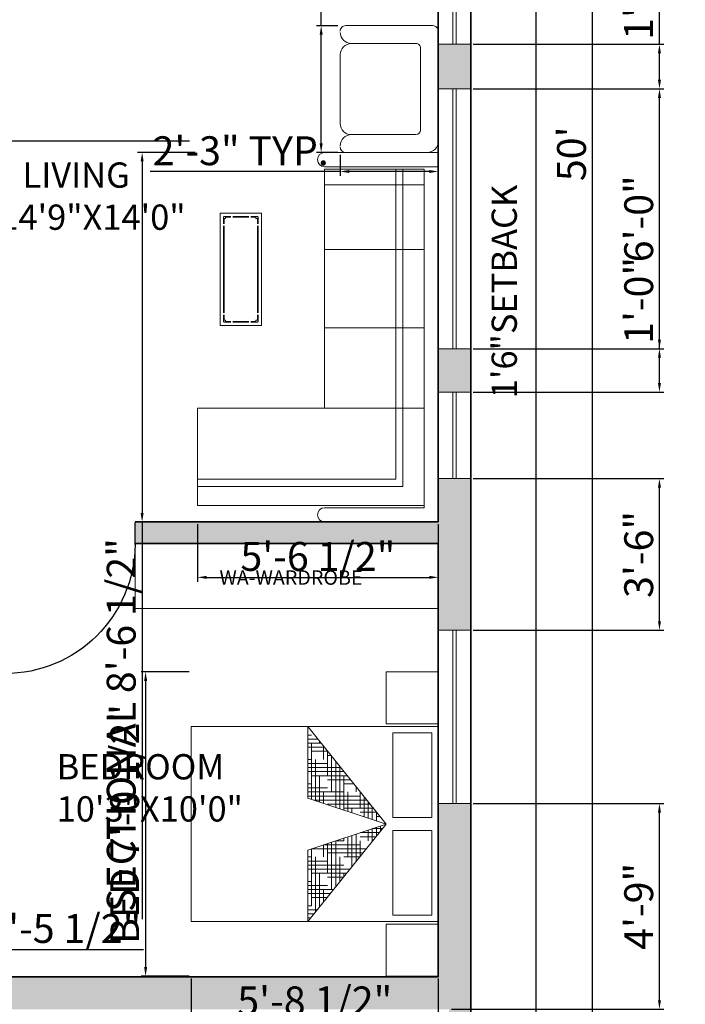
# Model space of a CAD drawing. Units: inches. Extents: x 2642 to 4124, y 1227 to 1973.
# Tile 3 of 7: x 3556 to 3741, y 1372 to 1645. Entities that reach past the tile are written whole.
import ezdxf

# ---------------------------------------------------------------- set-up
doc = ezdxf.new("R2010")
doc.units = ezdxf.units.IN
for name, color, linetype, lineweight in [('A-ANNO-DIMS', 2, 'Continuous', 18), ('A-ANNO-TEXT', 7, 'Continuous', 18), ('A-AREA-IDEN', 7, 'Continuous', 18), ('A-DOOR', 3, 'Continuous', 25), ('A-FLOR-CASE', 8, 'Continuous', 18), ('A-WALL', 7, 'Continuous', 35), ('A-WALL-PATT', 7, 'Continuous', 13), ('C-PROP', 7, 'Continuous', 25), ('furn', 165, 'Continuous', 18), ('window', 4, 'Continuous', 18)]:
    doc.layers.add(name, color=color, linetype=linetype, lineweight=lineweight)
doc.styles.get("Standard").update_dxf_attribs({"font": 'arial.ttf'})
doc.dimstyles.new('ISO-25', dxfattribs={"dimtxt": 8, "dimasz": 2.5, "dimexe": 1.25, "dimexo": 0.625, "dimtad": 1, "dimdec": 0, "dimlunit": 3, "dimtxsty": 'Standard', "dimcen": 2.5, "dimadec": 0, "dimazin": 0, "dimtfac": 1, "dimtdec": 0, "dimtmove": 0, "dimatfit": 3, "dimfxl": 1, "dimarcsym": 0})

# ---------------------------------------------------------------- blocks, each defined once
blk = doc.blocks.new('*D2')
at = {"layer": 'A-ANNO-DIMS', "color": 0, "lineweight": -2, "transparency": 16777216}
for p, q in [((3699.85, 1907.78), (3716.14, 1907.78)), ((3714.89, 1905.28), (3714.89, 1310.28)), ((3699.85, 1307.78), (3716.14, 1307.78))]:
    blk.add_line(p, q, dxfattribs=at)
at = {"layer": 'A-ANNO-DIMS', "color": 0, "transparency": 16777216}
for points in [[(3714.47, 1905.28), (3715.3, 1905.28), (3714.89, 1907.78)], [(3714.47, 1310.28), (3715.3, 1310.28), (3714.89, 1307.78)]]:
    blk.add_solid(points, dxfattribs=at)
at = {"layer": 'Defpoints', "color": 0, "transparency": 16777216}
for p in [(3699.22, 1907.78), (3699.22, 1307.78), (3714.89, 1307.78)]:
    blk.add_point(p, dxfattribs=at)
at = {"layer": 'A-ANNO-DIMS', "color": 0, "transparency": 16777216, "insert": (3710.18, 1607.78), "char_height": 8, "attachment_point": 5, "rotation": 90}
blk.add_mtext("50'", dxfattribs=at)
blk = doc.blocks.new('*U10')
for p, q in [((0, 0), (0, -6)), ((36, 0), (36, -6))]:
    blk.add_line(p, q)
blk.add_lwpolyline([(0, 0), (0, 36), (1.75, 36), (1.75, 0)], close=True)
blk.add_arc((0, 0), 36, 0, 90)
blk = doc.blocks.new('TABLE-30A')
at = {"color": 0, "linetype": 'ByBlock'}
for p, q in [((0, 0), (0, 0.55)), ((0, 0.55), (1.5, 0.55)), ((1.5, 0.55), (1.5, 0)), ((0.051, 0.508), (0.042, 0.499)), ((0.042, 0.499), (0.042, 0.478)), ((0.042, 0.478), (0.072, 0.478)), ((0.042, 0.478), (0.042, 0.41)), ((0.072, 0.508), (0.051, 0.508)), ((0.051, 0.478), (0.051, 0.41)), ((0.072, 0.478), (0.072, 0.508)), ((0.072, 0.508), (0.14, 0.508)), ((0.072, 0.499), (0.14, 0.499)), ((1.331, 0.508), (0.169, 0.508)), ((1.331, 0.499), (0.169, 0.499)), ((1.428, 0.508), (1.36, 0.508)), ((1.428, 0.499), (1.36, 0.499)), ((1.428, 0.508), (1.428, 0.478)), ((1.449, 0.508), (1.428, 0.508)), ((1.428, 0.478), (1.458, 0.478)), ((1.458, 0.499), (1.449, 0.508)), ((1.449, 0.478), (1.449, 0.41)), ((1.458, 0.478), (1.458, 0.499)), ((1.458, 0.478), (1.458, 0.41)), ((0.042, 0.169), (0.042, 0.381)), ((0.051, 0.169), (0.051, 0.381)), ((1.449, 0.381), (1.449, 0.169)), ((1.458, 0.381), (1.458, 0.169)), ((0.042, 0.072), (0.042, 0.14)), ((0.051, 0.072), (0.051, 0.14)), ((1.449, 0.072), (1.449, 0.14)), ((1.458, 0.072), (1.458, 0.14)), ((1.5, 0), (0, 0)), ((0.042, 0.072), (0.042, 0.051)), ((0.072, 0.072), (0.042, 0.072)), ((0.042, 0.051), (0.051, 0.042)), ((0.051, 0.042), (0.072, 0.042)), ((0.072, 0.042), (0.072, 0.072)), ((0.072, 0.051), (0.14, 0.051)), ((0.072, 0.042), (0.14, 0.042)), ((0.169, 0.051), (1.331, 0.051)), ((0.169, 0.042), (1.331, 0.042)), ((1.428, 0.051), (1.36, 0.051)), ((1.428, 0.042), (1.36, 0.042)), ((1.428, 0.072), (1.428, 0.042)), ((1.458, 0.072), (1.428, 0.072)), ((1.428, 0.042), (1.449, 0.042)), ((1.449, 0.042), (1.458, 0.051)), ((1.458, 0.051), (1.458, 0.072))]:
    blk.add_line(p, q, dxfattribs=at)
blk = doc.blocks.new('12')
at = {"color": 0}
for p, q in [((5656.26, 3021.25), (5553.9, 3021.25)), ((5553.9, 3021.25), (5553.9, 2989.76)), ((5557.83, 3021.25), (5557.83, 2989.76)), ((5656.26, 2989.76), (5656.26, 3021.25)), ((5652.32, 3017.31), (5558.49, 3017.31)), ((5558.49, 3017.31), (5558.49, 2989.76)), ((5562.89, 3017.31), (5562.89, 2989.76)), ((5580.8, 3017.31), (5580.8, 2989.76)), ((5602.45, 3017.31), (5602.45, 2989.76)), ((5624.76, 3017.31), (5624.76, 2954.53)), ((5651.66, 3017.31), (5651.66, 2954.53)), ((5652.32, 2989.76), (5652.32, 3017.31)), ((5646.42, 3011.41), (5558.49, 3011.41)), ((5644.45, 3009.44), (5558.49, 3009.44)), ((5644.45, 2954.53), (5644.45, 3009.44)), ((5646.42, 2954.53), (5646.42, 3011.41)), ((5624.76, 2995), (5624.76, 2954.53)), ((5558.49, 2989.76), (5624.76, 2989.76)), ((5651.66, 2954.53), (5624.76, 2954.53))]:
    blk.add_line(p, q, dxfattribs=at)
for centre in [(5555.86, 2989.76), (5654.29, 2989.76)]:
    blk.add_arc(centre, 1.97, 180, 0, dxfattribs=at)
at = {"xscale": -20.70834898381633, "yscale": 20.70834898381633, "zscale": 20.70834898381633}
blk.add_blockref('TABLE-30A', (5601.8, 2960.82), dxfattribs=at)
blk = doc.blocks.new('sofa-27')
at = {"color": 0, "linetype": 'ByBlock'}
for p, q in [((-0.0591, 0.0591), (-0.0591, 0.4902)), ((0.0945, 0.5198), (0.459, 0.5198)), ((0.6125, 0.0295), (0.6125, 0.4902)), ((0.0354, 0.1181), (0.0354, 0.4607)), ((0.518, 0.1181), (0.518, 0.4607)), ((0.4944, 0.0945), (0.0591, 0.0945)), ((0.583, 0), (0, 0))]:
    blk.add_line(p, q, dxfattribs=at)
for centre, radius, start, end in [((-0.0295, 0.4902), 0.0295, 90, 180), ((-0.0236, 0.4607), 0.0591, 360, 90), ((0.0945, 0.4607), 0.0591, 90, 180), ((0.459, 0.4607), 0.0591, 0, 90), ((0.5771, 0.4607), 0.0591, 90, 180), ((0.583, 0.4902), 0.0295, 0, 90), ((0.0591, 0.1181), 0.0236, 180, 270), ((0.4944, 0.1181), 0.0236, 270, 0), ((0, 0.0591), 0.0591, 180, 270), ((0.583, 0.0295), 0.0295, 270, 0)]:
    blk.add_arc(centre, radius, start, end, dxfattribs=at)
blk = doc.blocks.new('*X25')
at = {"color": 0}
for p, q in [((20.1875, 14.75), (20.1875, 14.7669)), ((20.199, 14.7812), (20.2772, 14.7812)), ((20.25, 14.8125), (20.2772, 14.8125)), ((20.1236, 14.6875), (20.25, 14.6875)), ((20.125, 14.5), (20.125, 14.6893)), ((20.1487, 14.7188), (20.2772, 14.7188)), ((20.1562, 14.625), (20.1562, 14.7281)), ((20.1739, 14.75), (20.2772, 14.75)), ((20.25, 14.3194), (20.25, 14.75)), ((20.0625, 14.2573), (20.0625, 14.6116)), ((20.0938, 14.375), (20.0938, 14.6504)), ((20.0984, 14.6562), (20.125, 14.6562)), ((20.2188, 14.3091), (20.2188, 14.625)), ((20.25, 14.625), (20.2772, 14.625)), ((20.023, 14.5625), (20.2772, 14.5625)), ((20.0312, 14.2469), (20.0312, 14.5727)), ((20.125, 14.5938), (20.2772, 14.5938)), ((19.9476, 14.4688), (20.125, 14.4688)), ((19.9727, 14.5), (20.25, 14.5)), ((19.9979, 14.5312), (20.2772, 14.5312)), ((20, 14.2366), (20, 14.5)), ((20.1875, 14.2987), (20.1875, 14.5)), ((19.9062, 14.375), (19.9062, 14.4174)), ((19.9225, 14.4375), (20, 14.4375)), ((20.125, 14.4062), (20.2772, 14.4062)), ((20.25, 14.4375), (20.2772, 14.4375)), ((19.8219, 14.3125), (20.2291, 14.3125)), ((19.8438, 14.1848), (19.8438, 14.3397)), ((19.875, 14.25), (19.875, 14.3785)), ((19.875, 14.3438), (20.2772, 14.3438)), ((19.9688, 14.2262), (19.9688, 14.375)), ((20, 14.375), (20.2772, 14.375)), ((20.1562, 14.2884), (20.1562, 14.375)), ((19.7716, 14.25), (20, 14.25)), ((19.7812, 14.1641), (19.7812, 14.262)), ((19.7967, 14.2812), (20.125, 14.2812)), ((19.8125, 14.1744), (19.8125, 14.3008)), ((19.9375, 14.2159), (19.9375, 14.25)), ((19.7213, 14.1875), (19.75, 14.1875)), ((19.7465, 14.2188), (19.875, 14.2188)), ((19.75, 14.1537), (19.75, 14.2231)), ((19.7018, 14.0938), (19.7786, 14.0938)), ((19.7188, 14.0726), (19.7188, 14.1136)), ((19.75, 14.0338), (19.75, 14.1032)), ((19.7812, 13.9949), (19.7812, 14.0929)), ((19.8125, 14), (19.8125, 14.0825)), ((19.7269, 14.0625), (19.8728, 14.0625)), ((19.752, 14.0312), (19.875, 14.0312)), ((19.9062, 13.8396), (19.9062, 14.0514)), ((19.9375, 13.8007), (19.9375, 14.0411)), ((19.9688, 13.875), (19.9688, 14.0307)), ((20, 14), (20, 14.0204)), ((19.8275, 13.9375), (20.25, 13.9375)), ((19.875, 13.8784), (19.875, 14)), ((19.875, 13.9688), (20.1557, 13.9688)), ((20, 14), (20.0614, 14)), ((20.0625, 13.6454), (20.0625, 13.9996)), ((20.0938, 13.625), (20.0938, 13.9893)), ((20.125, 13.75), (20.125, 13.9789)), ((20.1562, 13.875), (20.1562, 13.9686)), ((20.25, 13.5), (20.25, 13.9375)), ((19.8526, 13.9062), (20.125, 13.9062)), ((19.8777, 13.875), (20, 13.875)), ((20.0312, 13.6842), (20.0312, 13.875)), ((20.2188, 13.4511), (20.2188, 13.875)), ((20.25, 13.875), (20.2772, 13.875)), ((19.9532, 13.7812), (20.2772, 13.7812)), ((20, 13.8125), (20.2772, 13.8125)), ((20.125, 13.8438), (20.2772, 13.8438)), ((19.9783, 13.75), (20.25, 13.75)), ((20, 13.723), (20, 13.75)), ((20.0035, 13.7188), (20.125, 13.7188)), ((20.1875, 13.49), (20.1875, 13.75)), ((20.125, 13.6562), (20.2772, 13.6562)), ((20.25, 13.6875), (20.2772, 13.6875)), ((20.0789, 13.625), (20.2772, 13.625)), ((20.104, 13.5938), (20.2772, 13.5938)), ((20.1292, 13.5625), (20.25, 13.5625)), ((20.1562, 13.5288), (20.1562, 13.625)), ((20.25, 13.5), (20.2772, 13.5)), ((20.2046, 13.4688), (20.2772, 13.4688)), ((20.2297, 13.4375), (20.2772, 13.4375)), ((20.2549, 13.4062), (20.2772, 13.4062))]:
    blk.add_line(p, q, dxfattribs=at)
blk = doc.blocks.new('MAT-P02')
for p, q in [((-1.17, 0), (-1.17, -0.4)), ((-1.17, 0), (-0.77, 0)), ((-0.77, 0), (-0.77, -0.4)), ((-0.75, 0), (0.75, 0)), ((-0.75, 0), (-0.75, -1.9)), ((0.75, 0), (0.75, -1.9)), ((0.77, 0), (1.17, 0)), ((0.77, 0), (0.77, -0.4)), ((1.17, 0), (1.17, -0.4)), ((-0.7, -0.05), (-0.7, -0.35)), ((-0.7, -0.05), (-0.05, -0.05)), ((-0.05, -0.35), (-0.05, -0.05)), ((0.05, -0.05), (0.7, -0.05)), ((0.05, -0.35), (0.05, -0.05)), ((0.7, -0.05), (0.7, -0.35)), ((-0.7, -0.35), (-0.05, -0.35)), ((0.05, -0.35), (0.7, -0.35)), ((-1.17, -0.4), (-0.77, -0.4)), ((-0.75, -1.0034), (0, -0.4)), ((0, -0.4), (-0.75, -1.0034)), ((0, -0.4), (-0.2, -1.0034)), ((0, -0.4), (0.2, -1.0034)), ((0, -0.4), (0.75, -1.0034)), ((0.77, -0.4), (1.17, -0.4)), ((-0.75, -1.0034), (-0.2, -1.0034)), ((0.2, -1.0034), (0.75, -1.0034)), ((0.75, -1.9), (-0.75, -1.9))]:
    blk.add_line(p, q)
at = {"xscale": -1, "rotation": 90}
blk.add_blockref('*X25', (14.1285, 19.2738), dxfattribs=at)
blk = doc.blocks.new('WIN-24IN')
for p, q in [((0, 24), (9, 24)), ((4, 24), (4, 0)), ((5, 24), (5, 0)), ((0, 0), (9, 0))]:
    blk.add_line(p, q)
blk = doc.blocks.new('WIN-48IN')
for p, q in [((9, 48), (0, 48)), ((4, 48), (4, 0)), ((5, 48), (5, 0)), ((9, 0), (0, 0))]:
    blk.add_line(p, q)
blk = doc.blocks.new('*D40')
at = {"layer": 'A-ANNO-DIMS', "color": 0, "lineweight": -2, "transparency": 16777216}
for p, q in [((3639.76, 1643.28), (3639.76, 1765.19)), ((3644.41, 1643.28), (3638.51, 1643.28)), ((3639.76, 1610.65), (3639.76, 1640.78)), ((3644.41, 1608.15), (3638.51, 1608.15))]:
    blk.add_line(p, q, dxfattribs=at)
at = {"layer": 'A-ANNO-DIMS', "color": 0, "transparency": 16777216}
for points in [[(3639.34, 1640.78), (3640.18, 1640.78), (3639.76, 1643.28)], [(3639.34, 1610.65), (3640.18, 1610.65), (3639.76, 1608.15)]]:
    blk.add_solid(points, dxfattribs=at)
at = {"layer": 'Defpoints', "color": 0, "transparency": 16777216}
for p in [(3639.76, 1643.28), (3645.03, 1643.28), (3645.03, 1608.15)]:
    blk.add_point(p, dxfattribs=at)
at = {"layer": 'A-ANNO-DIMS', "color": 0, "transparency": 16777216, "insert": (3635, 1705.48), "char_height": 8, "attachment_point": 5, "rotation": 90}
blk.add_mtext('ARMCHAIR 2\'-11" TYP.', dxfattribs=at)
blk = doc.blocks.new('*D41')
at = {"layer": 'A-ANNO-DIMS', "color": 0, "lineweight": -2, "transparency": 16777216}
for p, q in [((3645.03, 1607.52), (3645.03, 1601.63)), ((3672.22, 1607.52), (3672.22, 1601.63)), ((3645.03, 1602.88), (3592.38, 1602.88)), ((3669.72, 1602.88), (3647.53, 1602.88))]:
    blk.add_line(p, q, dxfattribs=at)
at = {"layer": 'A-ANNO-DIMS', "color": 0, "transparency": 16777216}
for points in [[(3647.53, 1603.29), (3647.53, 1602.46), (3645.03, 1602.88)], [(3669.72, 1603.29), (3669.72, 1602.46), (3672.22, 1602.88)]]:
    blk.add_solid(points, dxfattribs=at)
at = {"layer": 'Defpoints', "color": 0, "transparency": 16777216}
for p in [(3645.03, 1608.15), (3672.22, 1608.15), (3645.03, 1602.88)]:
    blk.add_point(p, dxfattribs=at)
at = {"layer": 'A-ANNO-DIMS', "color": 0, "transparency": 16777216, "insert": (3617.46, 1607.59), "char_height": 8, "attachment_point": 5}
blk.add_mtext('2\'-3" TYP.', dxfattribs=at)
blk = doc.blocks.new('*D52')
at = {"layer": 'A-ANNO-DIMS', "color": 0, "lineweight": -2, "transparency": 16777216}
for p, q in [((3604.87, 1608.15), (3588.89, 1608.15)), ((3590.14, 1605.65), (3590.14, 1508.28)), ((3604.87, 1505.78), (3588.89, 1505.78)), ((3590.14, 1505.78), (3590.14, 1395.71))]:
    blk.add_line(p, q, dxfattribs=at)
at = {"layer": 'A-ANNO-DIMS', "color": 0, "transparency": 16777216}
for points in [[(3589.72, 1605.65), (3590.56, 1605.65), (3590.14, 1608.15)], [(3589.72, 1508.28), (3590.56, 1508.28), (3590.14, 1505.78)]]:
    blk.add_solid(points, dxfattribs=at)
at = {"layer": 'Defpoints', "color": 0, "transparency": 16777216}
for p in [(3605.5, 1608.15), (3590.14, 1505.78), (3605.5, 1505.78)]:
    blk.add_point(p, dxfattribs=at)
at = {"layer": 'A-ANNO-DIMS', "color": 0, "transparency": 16777216, "insert": (3585.38, 1449.5), "char_height": 8, "attachment_point": 5, "rotation": 90}
blk.add_mtext('SECTIONAL 8\'-6 1/2"', dxfattribs=at)
blk = doc.blocks.new('*D53')
at = {"layer": 'A-ANNO-DIMS', "color": 0, "lineweight": -2, "transparency": 16777216}
for p, q in [((3605.5, 1505.16), (3605.5, 1489.18)), ((3672.22, 1505.16), (3672.22, 1489.18)), ((3608, 1490.43), (3669.72, 1490.43))]:
    blk.add_line(p, q, dxfattribs=at)
at = {"layer": 'A-ANNO-DIMS', "color": 0, "transparency": 16777216}
for points in [[(3608, 1490.85), (3608, 1490.01), (3605.5, 1490.43)], [(3669.72, 1490.85), (3669.72, 1490.01), (3672.22, 1490.43)]]:
    blk.add_solid(points, dxfattribs=at)
at = {"layer": 'Defpoints', "color": 0, "transparency": 16777216}
for p in [(3605.5, 1505.78), (3672.22, 1505.78), (3672.22, 1490.43)]:
    blk.add_point(p, dxfattribs=at)
at = {"layer": 'A-ANNO-DIMS', "color": 0, "transparency": 16777216, "insert": (3638.86, 1495.19), "char_height": 8, "attachment_point": 5}
blk.add_mtext('5\'-6 1/2"', dxfattribs=at)
blk = doc.blocks.new('*D54')
at = {"layer": 'A-ANNO-DIMS', "color": 0, "lineweight": -2, "transparency": 16777216}
for p, q in [((3603.13, 1464.26), (3589.85, 1464.26)), ((3591.1, 1461.76), (3591.1, 1382.43)), ((3603.13, 1379.93), (3589.85, 1379.93))]:
    blk.add_line(p, q, dxfattribs=at)
at = {"layer": 'A-ANNO-DIMS', "color": 0, "transparency": 16777216}
for points in [[(3590.69, 1461.76), (3591.52, 1461.76), (3591.1, 1464.26)], [(3590.69, 1382.43), (3591.52, 1382.43), (3591.1, 1379.93)]]:
    blk.add_solid(points, dxfattribs=at)
at = {"layer": 'Defpoints', "color": 0, "transparency": 16777216}
for p in [(3603.75, 1464.26), (3591.1, 1379.93), (3603.75, 1379.93)]:
    blk.add_point(p, dxfattribs=at)
at = {"layer": 'A-ANNO-DIMS', "color": 0, "transparency": 16777216, "insert": (3586.34, 1422.09), "char_height": 8, "attachment_point": 5, "rotation": 90}
blk.add_mtext('BED 7\'-0 1/2"', dxfattribs=at)
blk = doc.blocks.new('*D55')
at = {"layer": 'A-ANNO-DIMS', "color": 0, "lineweight": -2, "transparency": 16777216}
for p, q in [((3603.75, 1379.31), (3603.75, 1366.03)), ((3672.22, 1379.31), (3672.22, 1366.03)), ((3606.25, 1367.28), (3669.72, 1367.28))]:
    blk.add_line(p, q, dxfattribs=at)
at = {"layer": 'A-ANNO-DIMS', "color": 0, "transparency": 16777216}
for points in [[(3606.25, 1367.7), (3606.25, 1366.87), (3603.75, 1367.28)], [(3669.72, 1367.7), (3669.72, 1366.87), (3672.22, 1367.28)]]:
    blk.add_solid(points, dxfattribs=at)
at = {"layer": 'Defpoints', "color": 0, "transparency": 16777216}
for p in [(3603.75, 1379.93), (3672.22, 1379.93), (3672.22, 1367.28)]:
    blk.add_point(p, dxfattribs=at)
at = {"layer": 'A-ANNO-DIMS', "color": 0, "transparency": 16777216, "insert": (3637.99, 1372.04), "char_height": 8, "attachment_point": 5}
blk.add_mtext('5\'-8 1/2"', dxfattribs=at)
blk = doc.blocks.new('*D64')
at = {"layer": 'A-ANNO-DIMS', "color": 0, "lineweight": -2, "transparency": 16777216}
for p, q in [((3495.22, 1391.16), (3495.22, 1386.09)), ((3524.83, 1391.16), (3524.83, 1386.09)), ((3497.72, 1387.34), (3522.33, 1387.34)), ((3524.83, 1387.34), (3590.54, 1387.34))]:
    blk.add_line(p, q, dxfattribs=at)
at = {"layer": 'A-ANNO-DIMS', "color": 0, "transparency": 16777216}
for points in [[(3497.72, 1387.76), (3497.72, 1386.93), (3495.22, 1387.34)], [(3522.33, 1387.76), (3522.33, 1386.93), (3524.83, 1387.34)]]:
    blk.add_solid(points, dxfattribs=at)
at = {"layer": 'Defpoints', "color": 0, "transparency": 16777216}
for p in [(3495.22, 1391.78), (3524.83, 1391.78), (3524.83, 1387.34)]:
    blk.add_point(p, dxfattribs=at)
at = {"layer": 'A-ANNO-DIMS', "color": 0, "transparency": 16777216, "insert": (3558.93, 1392.1), "char_height": 8, "attachment_point": 5}
blk.add_mtext('WC 2\'-5 1/2"', dxfattribs=at)
blk = doc.blocks.new('*D74')
at = {"layer": 'A-ANNO-DIMS', "color": 0, "lineweight": -2, "transparency": 16777216}
for p, q in [((3681.85, 1427.78), (3734.77, 1427.78)), ((3733.52, 1373.28), (3733.52, 1425.28)), ((3675.85, 1370.78), (3734.77, 1370.78))]:
    blk.add_line(p, q, dxfattribs=at)
at = {"layer": 'A-ANNO-DIMS', "color": 0, "transparency": 16777216}
for points in [[(3733.11, 1425.28), (3733.94, 1425.28), (3733.52, 1427.78)], [(3733.11, 1373.28), (3733.94, 1373.28), (3733.52, 1370.78)]]:
    blk.add_solid(points, dxfattribs=at)
at = {"layer": 'Defpoints', "color": 0, "transparency": 16777216}
for p in [(3681.22, 1427.78), (3733.52, 1427.78), (3675.22, 1370.78)]:
    blk.add_point(p, dxfattribs=at)
at = {"layer": 'A-ANNO-DIMS', "color": 0, "transparency": 16777216, "insert": (3728.81, 1399.28), "char_height": 8, "attachment_point": 5, "rotation": 90}
blk.add_mtext('4\'-9"', dxfattribs=at)
blk = doc.blocks.new('*D75')
at = {"layer": 'A-ANNO-DIMS', "color": 0, "lineweight": -2, "transparency": 16777216}
for p, q in [((3681.85, 1517.78), (3734.77, 1517.78)), ((3733.52, 1478.28), (3733.52, 1515.28)), ((3681.85, 1475.78), (3734.77, 1475.78))]:
    blk.add_line(p, q, dxfattribs=at)
at = {"layer": 'A-ANNO-DIMS', "color": 0, "transparency": 16777216}
for points in [[(3733.11, 1515.28), (3733.94, 1515.28), (3733.52, 1517.78)], [(3733.11, 1478.28), (3733.94, 1478.28), (3733.52, 1475.78)]]:
    blk.add_solid(points, dxfattribs=at)
at = {"layer": 'Defpoints', "color": 0, "transparency": 16777216}
for p in [(3681.22, 1517.78), (3733.52, 1517.78), (3681.22, 1475.78)]:
    blk.add_point(p, dxfattribs=at)
at = {"layer": 'A-ANNO-DIMS', "color": 0, "transparency": 16777216, "insert": (3728.81, 1496.78), "char_height": 8, "attachment_point": 5, "rotation": 90}
blk.add_mtext('3\'-6"', dxfattribs=at)
blk = doc.blocks.new('*D76')
at = {"layer": 'A-ANNO-DIMS', "color": 0, "lineweight": -2, "transparency": 16777216}
for p, q in [((3733.52, 1553.78), (3733.52, 1578.05)), ((3681.85, 1553.78), (3734.77, 1553.78)), ((3733.52, 1544.28), (3733.52, 1551.28)), ((3681.85, 1541.78), (3734.77, 1541.78))]:
    blk.add_line(p, q, dxfattribs=at)
at = {"layer": 'A-ANNO-DIMS', "color": 0, "transparency": 16777216}
for points in [[(3733.11, 1551.28), (3733.94, 1551.28), (3733.52, 1553.78)], [(3733.11, 1544.28), (3733.94, 1544.28), (3733.52, 1541.78)]]:
    blk.add_solid(points, dxfattribs=at)
at = {"layer": 'Defpoints', "color": 0, "transparency": 16777216}
for p in [(3681.22, 1553.78), (3733.52, 1553.78), (3681.22, 1541.78)]:
    blk.add_point(p, dxfattribs=at)
at = {"layer": 'A-ANNO-DIMS', "color": 0, "transparency": 16777216, "insert": (3728.81, 1567.16), "char_height": 8, "attachment_point": 5, "rotation": 90}
blk.add_mtext('1\'-0"', dxfattribs=at)
blk = doc.blocks.new('*D77')
at = {"layer": 'A-ANNO-DIMS', "color": 0, "lineweight": -2, "transparency": 16777216}
for p, q in [((3681.85, 1625.78), (3734.77, 1625.78)), ((3733.52, 1556.28), (3733.52, 1623.28)), ((3681.85, 1553.78), (3734.77, 1553.78))]:
    blk.add_line(p, q, dxfattribs=at)
at = {"layer": 'A-ANNO-DIMS', "color": 0, "transparency": 16777216}
for points in [[(3733.11, 1623.28), (3733.94, 1623.28), (3733.52, 1625.78)], [(3733.11, 1556.28), (3733.94, 1556.28), (3733.52, 1553.78)]]:
    blk.add_solid(points, dxfattribs=at)
at = {"layer": 'Defpoints', "color": 0, "transparency": 16777216}
for p in [(3681.22, 1625.78), (3733.52, 1625.78), (3681.22, 1553.78)]:
    blk.add_point(p, dxfattribs=at)
at = {"layer": 'A-ANNO-DIMS', "color": 0, "transparency": 16777216, "insert": (3728.81, 1589.78), "char_height": 8, "attachment_point": 5, "rotation": 90}
blk.add_mtext('6\'-0"', dxfattribs=at)
blk = doc.blocks.new('*D78')
at = {"layer": 'A-ANNO-DIMS', "color": 0, "lineweight": -2, "transparency": 16777216}
for p, q in [((3733.52, 1638.12), (3733.52, 1681.02)), ((3681.85, 1638.12), (3734.77, 1638.12)), ((3733.52, 1628.28), (3733.52, 1635.62)), ((3681.85, 1625.78), (3734.77, 1625.78))]:
    blk.add_line(p, q, dxfattribs=at)
at = {"layer": 'A-ANNO-DIMS', "color": 0, "transparency": 16777216}
for points in [[(3733.11, 1635.62), (3733.94, 1635.62), (3733.52, 1638.12)], [(3733.11, 1628.28), (3733.94, 1628.28), (3733.52, 1625.78)]]:
    blk.add_solid(points, dxfattribs=at)
at = {"layer": 'Defpoints', "color": 0, "transparency": 16777216}
for p in [(3681.22, 1638.12), (3733.52, 1638.12), (3681.22, 1625.78)]:
    blk.add_point(p, dxfattribs=at)
at = {"layer": 'A-ANNO-DIMS', "color": 0, "transparency": 16777216, "insert": (3728.76, 1660.82), "char_height": 8, "attachment_point": 5, "rotation": 90}
blk.add_mtext('1\'-0 1/2"', dxfattribs=at)
blk = doc.blocks.new('*D83')
at = {"layer": 'A-ANNO-DIMS', "color": 0, "lineweight": -2, "transparency": 16777216}
for p, q in [((3413.99, 1611.28), (3493.83, 1611.28)), ((3603.25, 1611.28), (3496.33, 1611.28))]:
    blk.add_line(p, q, dxfattribs=at)
at = {"layer": 'A-ANNO-DIMS', "color": 0, "transparency": 16777216}
blk.add_solid([(3493.83, 1611.7), (3493.83, 1610.87), (3496.33, 1611.28)], dxfattribs=at)
at = {"layer": 'Defpoints', "color": 0, "transparency": 16777216}
for p in [(3496.33, 1611.28), (3603.25, 1611.28)]:
    blk.add_point(p, dxfattribs=at)
at = {"layer": 'A-ANNO-DIMS', "color": 0, "transparency": 16777216, "insert": (3432.18, 1615.99), "char_height": 8, "attachment_point": 5}
blk.add_mtext('R8\'-11"', dxfattribs=at)

msp = doc.modelspace()

# ---------------------------------------------------------------- hatches: boundary and pattern name
at = {"layer": 'A-WALL-PATT'}
h = msp.add_hatch(color=256, dxfattribs=at)
h.dxf.hatch_style = 1
h.paths.add_polyline_path([(3552.22, 1505.78), (3495.22, 1505.78), (3495.22, 1508.78), (3492.22, 1508.78), (3486.22, 1508.78), (3486.22, 1415.78), (3495.22, 1415.78), (3495.22, 1499.78), (3543.22, 1499.78), (3543.22, 1457.78), (3549.22, 1457.78), (3549.22, 1499.78), (3552.19, 1499.78), (3552.19, 1499.78)])
h.paths.add_polyline_path([(3681.22, 1427.78), (3672.22, 1427.78), (3672.22, 1395.07), (3672.22, 1379.78), (3549.22, 1379.78), (3549.22, 1427.78), (3543.22, 1427.78), (3543.22, 1379.78), (3495.22, 1379.78), (3495.22, 1391.78), (3486.22, 1391.78), (3486.22, 1370.78), (3675.22, 1370.78), (3675.22, 1307.78), (3681.22, 1307.78)])
h.paths.add_polyline_path([(3681.22, 1517.78), (3672.22, 1517.78), (3672.22, 1505.78), (3640.73, 1505.78), (3588.22, 1505.78), (3588.22, 1499.78), (3672.22, 1499.78), (3672.22, 1475.78), (3681.22, 1475.78)])
h.paths.add_polyline_path([(3681.22, 1638.12), (3672.22, 1638.12), (3672.22, 1625.78), (3681.22, 1625.78)])
h.paths.add_polyline_path([(3681.22, 1553.78), (3672.22, 1553.78), (3672.22, 1541.78), (3681.22, 1541.78)])
h.paths.add_polyline_path([(3528.22, 1844.78), (3552.22, 1844.78), (3552.22, 1847.78), (3552.22, 1853.78), (3519.22, 1853.78), (3519.22, 1682.78), (3486.22, 1682.78), (3486.22, 1548.78), (3492.22, 1548.78), (3495.22, 1548.78), (3495.22, 1673.78), (3528.22, 1673.78)])
h.paths.add_polyline_path([(3681.22, 1865.78), (3675.22, 1865.78), (3675.22, 1853.78), (3615.22, 1853.78), (3615.22, 1856.78), (3609.22, 1856.78), (3609.22, 1853.78), (3582.22, 1853.78), (3582.22, 1847.78), (3582.22, 1844.78), (3672.22, 1844.78), (3672.22, 1823.67), (3681.22, 1823.67)])
h.paths.add_polyline_path([(3681.22, 1907.78), (3519.22, 1907.78), (3519.22, 1901.78), (3540.68, 1901.78), (3609.22, 1901.78), (3609.22, 1886.78), (3615.22, 1886.78), (3615.22, 1901.78), (3675.22, 1901.78), (3675.22, 1889.78), (3681.22, 1889.78)])
h.paths.add_polyline_path([(3681.22, 1775.67), (3672.22, 1775.67), (3672.22, 1742.87), (3681.22, 1742.87)])
h.paths.add_polyline_path([(3681.22, 1694.87), (3672.22, 1694.87), (3672.22, 1682.78), (3600.22, 1682.78), (3600.22, 1673.78), (3672.22, 1673.78), (3672.22, 1662.12), (3681.22, 1662.12)])

# ---------------------------------------------------------------- linework, layer by layer
at = {"layer": 'A-FLOR-CASE'}
for p in [(3588.22, 1505.78), (3672.22, 1481.78)]:
    msp.add_line(p, (3588.22, 1481.78), dxfattribs=at)
at = {"layer": 'A-WALL'}
for p, q in [((3681.22, 1907.78), (3681.22, 1307.78)), ((3672.22, 1673.78), (3672.22, 1505.78)), ((3672.22, 1505.78), (3588.22, 1505.78)), ((3672.22, 1499.78), (3588.22, 1499.78)), ((3672.22, 1499.78), (3672.22, 1379.78)), ((3672.22, 1379.78), (3549.22, 1379.78))]:
    msp.add_line(p, q, dxfattribs=at)
at = {"layer": 'C-PROP'}
msp.add_line((3699.22, 1907.78), (3699.22, 1307.78), dxfattribs=at)
at = {"layer": 'window'}
for p, q in [((3681.22, 1625.78), (3672.22, 1625.78)), ((3676.22, 1625.78), (3676.22, 1553.78)), ((3677.22, 1625.78), (3677.22, 1553.78)), ((3681.22, 1553.78), (3672.22, 1553.78))]:
    msp.add_line(p, q, dxfattribs=at)

# ---------------------------------------------------------------- block references
at = {"layer": 'A-DOOR', "xscale": -1, "rotation": 179.6786649249896}
msp.add_blockref('*U10', (3552.19, 1499.78), dxfattribs=at)
at = {"layer": 'furn'}
for name, p, xscale, yscale, zscale, rotation in [('sofa-27', (3672.22, 1611.24), 52.31545737226423, 52.31545737226423, 52.31545737226423, 89.99999999999667), ('MAT-P02', (3672.22, 1422.09), 36.03633950593442, 36.03633950593442, 36.03633950593442, 270)]:
    msp.add_blockref(name, p, dxfattribs=dict(at, xscale=xscale, yscale=yscale, zscale=zscale, rotation=rotation))
at = {"layer": 'furn', "rotation": 270}
msp.add_blockref('12', (650.97, 7162.04), dxfattribs=at)
at = {"layer": 'window'}
for name, p in [('WIN-24IN', (3672.22, 1638.12)), ('WIN-24IN', (3672.22, 1517.78)), ('WIN-48IN', (3672.22, 1427.78))]:
    msp.add_blockref(name, p, dxfattribs=at)

# ---------------------------------------------------------------- texts
at = {"layer": 'A-ANNO-TEXT', "insert": (3687, 1540.05), "char_height": 7, "attachment_point": 1, "rotation": 90}
msp.add_mtext_dynamic_manual_height_columns('{\\fTimes New Roman|b0|i0|c0|p18;1\'6"SETBACK}', width=61.0557, gutter_width=12.5, heights=[0], dxfattribs=at)
at = {"layer": 'A-ANNO-TEXT', "insert": (3611.58, 1492.37), "char_height": 4, "attachment_point": 1}
msp.add_mtext_dynamic_manual_height_columns('WA-WARDROBE', width=29.5334, gutter_width=12.5, heights=[0], dxfattribs=at)
at = {"layer": 'A-AREA-IDEN', "char_height": 7, "attachment_point": 1}
for s, insert in [('{\\fTimes New Roman|b0|i0|c0|p18;   LIVING\\P14\'9"X14\'0"}', (3550.56, 1605.39)), ('{\\fTimes New Roman|b0|i0|c0|p18;BEDROOM\\P10\'3"X10\'0"}', (3566.45, 1441.45))]:
    msp.add_mtext_dynamic_manual_height_columns(s, width=61.0557, gutter_width=12.5, heights=[0], dxfattribs=dict(at, insert=insert))

# ---------------------------------------------------------------- dimensions: what is measured, and where the dimension line sits
at = {"layer": 'A-ANNO-DIMS'}
for base, p1, p2, override, picture, middle in [((3714.89, 1307.78), (3699.22, 1907.78), (3699.22, 1307.78), {"dimclrd": 0, "dimclre": 0, "dimclrt": 0}, '*D2', (3710.18, 1607.78)), ((3733.52, 1638.12), (3681.22, 1625.78), (3681.22, 1638.12), {"dimdec": 1, "dimlfac": 1, "dimrnd": 0, "dimzin": 1, "dimdsep": 46, "dimlunit": 4, "dimfrac": 2}, '*D78', (3728.76, 1660.82)), ((3733.52, 1625.78), (3681.22, 1553.78), (3681.22, 1625.78), {"dimdec": 1, "dimlfac": 1, "dimrnd": 0, "dimzin": 1, "dimdsep": 46, "dimlunit": 4, "dimfrac": 2}, '*D77', (3728.81, 1589.78)), ((3733.52, 1553.78), (3681.22, 1541.78), (3681.22, 1553.78), {"dimdec": 1, "dimlfac": 1, "dimrnd": 0, "dimzin": 1, "dimdsep": 46, "dimlunit": 4, "dimfrac": 2}, '*D76', (3728.81, 1567.16)), ((3733.52, 1517.78), (3681.22, 1475.78), (3681.22, 1517.78), {"dimdec": 1, "dimlfac": 1, "dimrnd": 0, "dimzin": 1, "dimdsep": 46, "dimlunit": 4, "dimfrac": 2}, '*D75', (3728.81, 1496.78)), ((3733.52, 1427.78), (3675.22, 1370.78), (3681.22, 1427.78), {"dimdec": 1, "dimlfac": 1, "dimrnd": 0, "dimzin": 1, "dimdsep": 46, "dimlunit": 4, "dimfrac": 2}, '*D74', (3728.81, 1399.28))]:
    dim = msp.add_linear_dim(base=base, p1=p1, p2=p2, angle=90, dimstyle='ISO-25', override=override, dxfattribs=at)
    dim.commit()
    dim.dimension.update_dxf_attribs({"geometry": picture, "text_midpoint": middle})
for base, p1, p2, angle, text, picture, middle in [((3639.76, 1643.28), (3645.03, 1608.15), (3645.03, 1643.28), 90, 'ARMCHAIR <> TYP.', '*D40', (3635, 1705.48)), ((3645.03, 1602.88), (3672.22, 1608.15), (3645.03, 1608.15), 180, '<> TYP.', '*D41', (3617.46, 1607.59)), ((3590.14, 1505.78), (3605.5, 1608.15), (3605.5, 1505.78), 270, 'SECTIONAL <>', '*D52', (3585.38, 1449.5)), ((3591.1, 1379.93), (3603.75, 1464.26), (3603.75, 1379.93), 270, 'BED <>', '*D54', (3586.34, 1422.09))]:
    dim = msp.add_linear_dim(base=base, p1=p1, p2=p2, angle=angle, text=text, dimstyle='ISO-25', override={"dimdec": 1, "dimlfac": 1, "dimrnd": 0, "dimzin": 1, "dimdsep": 46, "dimlunit": 4, "dimfrac": 2}, dxfattribs=at)
    dim.commit()
    dim.dimension.update_dxf_attribs({"geometry": picture, "text_midpoint": middle})
dim = msp.add_radius_dim(center=(3603.25, 1611.28), mpoint=(3496.33, 1611.28), dimstyle='ISO-25', override={"dimdec": 1, "dimlfac": 1, "dimrnd": 0, "dimzin": 1, "dimdsep": 46, "dimlunit": 4, "dimfrac": 2}, dxfattribs=at)
dim.commit()
dim.dimension.update_dxf_attribs({"geometry": '*D83', "text_midpoint": (3432.18, 1611.28), "dimtype": 164})
for base, p1, p2, picture, middle in [((3672.22, 1490.43), (3605.5, 1505.78), (3672.22, 1505.78), '*D53', (3638.86, 1495.19)), ((3672.22, 1367.28), (3603.75, 1379.93), (3672.22, 1379.93), '*D55', (3637.99, 1372.04))]:
    dim = msp.add_linear_dim(base=base, p1=p1, p2=p2, dimstyle='ISO-25', override={"dimdec": 1, "dimlfac": 1, "dimrnd": 0, "dimzin": 1, "dimdsep": 46, "dimlunit": 4, "dimfrac": 2}, dxfattribs=at)
    dim.commit()
    dim.dimension.update_dxf_attribs({"geometry": picture, "text_midpoint": middle})
dim = msp.add_linear_dim(base=(3524.83, 1387.34), p1=(3495.22, 1391.78), p2=(3524.83, 1391.78), text='WC <>', dimstyle='ISO-25', override={"dimdec": 1, "dimlfac": 1, "dimrnd": 0, "dimzin": 1, "dimdsep": 46, "dimlunit": 4, "dimfrac": 2}, dxfattribs=at)
dim.commit()
dim.dimension.update_dxf_attribs({"geometry": '*D64', "text_midpoint": (3558.93, 1392.1)})

doc.saveas('drawing.dxf')
